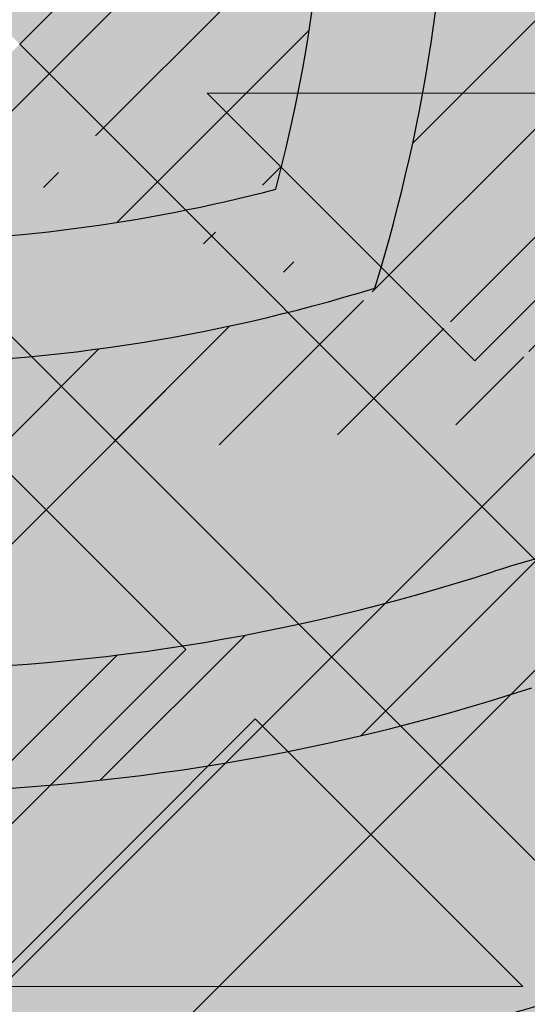
# Model space of a CAD drawing. Units: inches. Extents: x 844 to 2234, y 346 to 1084.
# Tile 10 of 93: x 1123.249 to 1124.57, y 688.619 to 691.183. Entities that reach past the tile are written whole.
import ezdxf

# ---------------------------------------------------------------- set-up
doc = ezdxf.new("R2010")
doc.units = ezdxf.units.IN
doc.header["$MEASUREMENT"] = 0
for name, color, linetype, lineweight in [('A-ANNO-DIMS', 2, 'Continuous', 18), ('furniture', 8, 'Continuous', 18), ('RA-AP-01$0$INT', 35, 'Continuous', 5)]:
    doc.layers.add(name, color=color, linetype=linetype, lineweight=lineweight)
doc.layers.add('RA-AP-01$0$FURN', color=3, linetype='Continuous')
doc.layers.add('RA-AP-01$0$WOOD', color=64, linetype='Continuous')
doc.styles.get("Standard").update_dxf_attribs({"font": 'arial.ttf'})
doc.dimstyles.get("Standard").update_dxf_attribs({"dimtxt": 6, "dimasz": 3, "dimexe": 0.18, "dimexo": 0.0625, "dimgap": 0.09, "dimtad": 0, "dimtih": 1, "dimtoh": 1, "dimdec": 1, "dimzin": 0, "dimdsep": 46, "dimlunit": 3, "dimtxsty": 'Standard', "dimblk": 'ARCHTICK', "dimcen": 0.09, "dimadec": 0, "dimazin": 0, "dimtfac": 1, "dimtdec": 1, "dimtofl": 0, "dimtmove": 0, "dimatfit": 3, "dimfxl": 1, "dimtolj": 1, "dimtzin": 0, "dimarcsym": 0})

# ---------------------------------------------------------------- blocks, each defined once
blk = doc.blocks.new('A$C18D01794')
at = {"layer": 'RA-AP-01$0$INT'}
h = blk.add_hatch(color=256, dxfattribs=at)
h.paths.add_polyline_path([(4.585917135068449, -6.356712009588271), (4.555206456959269, -6.35671200958746), (4.555206456959137, -6.387422687716308), (4.874495778835233, -6.706712009592356), (4.90520645695423, -6.676001331474049)])
h.paths.add_polyline_path([(5.255206456948813, -6.387422687716306), (5.255206456948682, -6.356712009605972), (5.224495778822613, -6.356712009605161), (4.905206456953498, -6.676001331474273), (4.935917135072151, -6.706712009592924)])
h.paths.add_polyline_path([(4.935917135072559, -6.706712009592068), (4.905206456953564, -6.737422687710376), (5.255206456951813, -7.087422687708613), (5.255206456951549, -7.026001331471008)])
h.paths.add_polyline_path([(4.555206456956399, -7.026001331471013), (4.555206456956134, -7.087422687708616), (4.905206456953821, -6.737422687710943), (4.874495778835166, -6.70671200959229)])
h = blk.add_hatch(color=256, dxfattribs=at)
h.paths.add_polyline_path([(4.585917135068448, -6.356712009588273), (4.614201406330596, -6.356712009589021), (4.668846067270487, -6.411356670531338), (4.723490728212344, -6.356712009591912), (4.771774999457151, -6.35671200959319), (4.826419660396886, -6.411356670535356), (4.862780050090322, -6.374996280843536), (4.844495778842715, -6.356712009595112), (4.862780050090411, -6.356712009595595), (4.905206456960182, -6.399138416468211), (4.947632863832445, -6.356712009597838), (4.965917135079675, -6.356712009598322), (4.947632863831759, -6.374996280845421), (4.983993253523576, -6.411356670538857), (5.038637914464627, -6.356712009600247), (5.08692218571208, -6.356712009601523), (5.141566846649976, -6.411356670541852), (5.196211507589851, -6.356712009604411), (5.224495778822615, -6.356712009605161), (4.905206456953975, -6.676001331473793)])
h.paths.add_polyline_path([(4.895206456956031, -6.637717060225675), (4.895206456958921, -6.528427738347902), (4.840561796018589, -6.583072399285802)], flags=16)
h.paths.add_polyline_path([(4.915206456955638, -6.637717060226121), (4.969851117895509, -6.583072399288678), (4.915206456957609, -6.528427738348344)], flags=16)
h.paths.add_polyline_path([(4.826419660395175, -6.568930263661755), (4.881064321335613, -6.514285602723745), (4.771774999456703, -6.514285602720857)], flags=16)
h.paths.add_polyline_path([(4.983993253519558, -6.568930263665262), (5.038637914460456, -6.514285602726792), (4.929348592581548, -6.514285602724816)], flags=16)
h.paths.add_polyline_path([(4.881064321336025, -6.494285602723742), (4.826419660397532, -6.439640941782821), (4.771774999457062, -6.494285602720859)], flags=16)
h.paths.add_polyline_path([(4.929348592582019, -6.494285602724817), (5.038637914460982, -6.494285602726792), (4.983993253522945, -6.439640941786327)], flags=16)
h.paths.add_polyline_path([(4.895206456960191, -6.480143467100443), (4.895206456962115, -6.407422687715913), (4.876922185715016, -6.389138416467584), (4.840561796021581, -6.425498806159401)], flags=16)
h.paths.add_polyline_path([(4.915206456958487, -6.480143467100889), (4.969851117899527, -6.425498806162279), (4.933490728206909, -6.389138416468043), (4.9152064569598, -6.40742268771434)], flags=16)
h.paths.add_polyline_path([(4.757632863832376, -6.480143467096812), (4.812277524772842, -6.425498806158772), (4.757632863834348, -6.370854145217844)], flags=16)
h.paths.add_polyline_path([(4.737632863832376, -6.480143467096286), (4.737632863834348, -6.370854145217375), (4.682988202893906, -6.425498806155385)], flags=16)
h.paths.add_polyline_path([(5.05278005008503, -6.480143467103376), (5.052780050087917, -6.370854145224413), (4.998135389146995, -6.425498806162908)], flags=16)
h.paths.add_polyline_path([(5.072780050085024, -6.480143467103744), (5.127424711025931, -6.42549880616527), (5.072780050087916, -6.370854145224832)], flags=16)
h.paths.add_polyline_path([(4.935917135072783, -6.706712009592292), (5.255206456948811, -6.387422687716309), (5.255206456948932, -6.415706958964177), (5.200561796010279, -6.470351619902839), (5.255206456949403, -6.524996280841948), (5.25520645694961, -6.5732805520894), (5.200561796009787, -6.627925213029239), (5.236922185702417, -6.664285602721864), (5.255206456949919, -6.646001331474357), (5.255206456949998, -6.664285602721898), (5.212780050078687, -6.706712009592262), (5.25520645695036, -6.749138416463932), (5.255206456950438, -6.767422687711313), (5.236922185702424, -6.749138416463297), (5.200561796009796, -6.785498806155928), (5.255206456950753, -6.840143467096874), (5.25520645695096, -6.888427738341682), (5.200561796010322, -6.943072399282328), (5.255206456951428, -6.997717060223427), (5.255206456951547, -7.026001331471006)])
h.paths.add_polyline_path([(5.042988202883395, -6.785498806155427), (5.097632863823085, -6.840143467095101), (5.097632863822622, -6.730854145216193)], flags=16)
h.paths.add_polyline_path([(5.028846067259663, -6.771356670531693), (5.083490728198774, -6.716712009592573), (4.974201406321001, -6.716712009593042)], flags=16)
h.paths.add_polyline_path([(5.117632863823087, -6.840143467095186), (5.172277524762331, -6.785498806155926), (5.11763286382262, -6.730854145216225)], flags=16)
h.paths.add_polyline_path([(5.08349072819877, -6.696712009593886), (5.028846067259652, -6.642067348654775), (4.974201406320998, -6.696712009593438)], flags=16)
h.paths.add_polyline_path([(5.131774999446817, -6.854285602718917), (5.186419660386065, -6.799640941779662), (5.241064321325782, -6.854285602719365)], flags=17)
h.paths.add_polyline_path([(5.131774999446228, -6.716712009592374), (5.186419660386065, -6.771356670532194), (5.222780050079488, -6.734996280838764), (5.204495778832781, -6.716712009592063)], flags=16)
h.paths.add_polyline_path([(5.097632863822613, -6.682569873970264), (5.097632863823061, -6.573280552091354), (5.042988202883383, -6.627925213031044)], flags=16)
h.paths.add_polyline_path([(5.131774999446899, -6.874285602718915), (5.241064321325809, -6.874285602719364), (5.186419660386591, -6.928930263658598)], flags=17)
h.paths.add_polyline_path([(5.131774999446226, -6.696712009594078), (5.204495778830767, -6.696712009594374), (5.22278005007868, -6.67842773834687), (5.186419660386049, -6.642067348654249)], flags=16)
h.paths.add_polyline_path([(5.11763286382262, -6.682569873970225), (5.17227752476232, -6.627925213030515), (5.117632863823064, -6.573280552091267)], flags=16)
h.paths.add_polyline_path([(5.186419660386069, -6.613783077405491), (5.241064321325754, -6.559138416465795), (5.131774999446791, -6.559138416466263)], flags=16)
h.paths.add_polyline_path([(5.131774999446872, -6.539138416466263), (5.24106432132578, -6.539138416465794), (5.186419660386554, -6.484493755526573)], flags=16)
h.paths.add_polyline_path([(5.255206456951811, -7.08742268770861), (5.255206456951895, -7.106712009588038), (4.555206456956052, -7.106712009588038), (4.555206456956136, -7.087422687708617), (4.905206456953973, -6.737422687710788)])
h.paths.add_polyline_path([(4.983993253513404, -6.8444937555241), (4.92934859257295, -6.899138416462108), (5.03863791445186, -6.899138416465014)], flags=16)
h.paths.add_polyline_path([(4.969851117889988, -6.83035161990006), (4.915206456952556, -6.775706958960171), (4.915206456949648, -6.884996280837944)], flags=16)
h.paths.add_polyline_path([(4.929348592572535, -6.919138416462105), (4.983993253511019, -6.973783077403037), (5.038637914451496, -6.919138416465012)], flags=16)
h.paths.add_polyline_path([(5.052780050074912, -6.93328055208906), (4.998135389134438, -6.987925213027088), (5.052780050072919, -7.042569873968025)], flags=16)
h.paths.add_polyline_path([(5.07278005007491, -6.933280552089588), (5.072780050072918, -7.042569873968497), (5.127424711013374, -6.987925213030498)], flags=16)
h.paths.add_polyline_path([(4.89520645695295, -6.775706958959721), (4.840561796013067, -6.830351619897157), (4.895206456950961, -6.884996280837494)], flags=16)
h.paths.add_polyline_path([(4.915206456948365, -6.933280552085403), (4.915206456946434, -7.006001331471951), (4.933490728192729, -7.024285602719066), (4.969851117886972, -6.987925213026453)], flags=16)
h.paths.add_polyline_path([(4.881064321327021, -6.899138416461022), (4.82641966038902, -6.84449375552057), (4.771774999448108, -6.899138416459029)], flags=16)
h.paths.add_polyline_path([(4.895206456950073, -6.933280552084951), (4.840561796009022, -6.987925213023558), (4.876922185700835, -7.024285602716997), (4.895206456948749, -7.006001331469487)], flags=16)
h.paths.add_polyline_path([(4.983993253510392, -7.0020673486505), (4.947632863816944, -7.038427738342319), (4.965917135064043, -7.05671200959023), (5.038637914448995, -7.056712009591555)], flags=16)
h.paths.add_polyline_path([(4.881064321326543, -6.91913841646102), (4.771774999447578, -6.919138416459031), (4.826419660385607, -6.973783077399508)], flags=16)
h.paths.add_polyline_path([(4.905206456946447, -7.014285602717636), (4.862780050074785, -7.056712009588352), (4.947632863816685, -7.056712009589775)], flags=16)
h.paths.add_polyline_path([(5.14156684663679, -7.002067348654549), (5.086922185696452, -7.056712009592438), (5.196211507574223, -7.056712009594425)], flags=16)
h.paths.add_polyline_path([(4.8264196603837, -7.002067348646972), (4.771774999442643, -7.056712009585575), (4.8444957788276, -7.056712009587508), (4.862780050075511, -7.038427738340416)], flags=16)
h.paths.add_polyline_path([(4.812277524760289, -6.98792521302292), (4.757632863822258, -6.933280552082447), (4.757632863819352, -7.042569873961408)], flags=16)
h.paths.add_polyline_path([(4.73763286382226, -6.933280552082079), (4.682988202881349, -6.987925213020536), (4.737632863819352, -7.04256987396099)], flags=16)
h.paths.add_polyline_path([(4.723490728195188, -7.056712009584289), (4.668846067257299, -7.002067348643949), (4.614201406317417, -7.056712009581383)], flags=16)
h.paths.add_polyline_path([(4.597632863829262, -6.706712009592262), (4.555206456957951, -6.664285602721896), (4.555206456958029, -6.646001331474357), (4.573490728205535, -6.664285602721864), (4.609851117898167, -6.627925213029238), (4.555206456958338, -6.573280552089402), (4.555206456958546, -6.524996280841952), (4.60985111789767, -6.470351619902839), (4.555206456959015, -6.415706958964177), (4.555206456959138, -6.387422687716309), (4.874495778835167, -6.70671200959229), (4.5552064569564, -7.026001331471015), (4.555206456956523, -6.997717060223433), (4.609851117897629, -6.94307239928233), (4.555206456956988, -6.888427738341681), (4.555206456957198, -6.840143467096881), (4.609851117898153, -6.78549880615593), (4.573490728205528, -6.749138416463297), (4.555206456957507, -6.76742268771132), (4.555206456957585, -6.749138416463933)])
h.paths.add_polyline_path([(4.712780050085332, -6.730854145216195), (4.712780050084863, -6.840143467095105), (4.767424711024555, -6.785498806155427)], flags=16)
h.paths.add_polyline_path([(4.726922185709173, -6.716712009592573), (4.781566846648288, -6.771356670531693), (4.836211507586949, -6.716712009593043)], flags=16)
h.paths.add_polyline_path([(4.692780050085327, -6.730854145216225), (4.638135389145619, -6.785498806155928), (4.692780050084865, -6.840143467095185)], flags=16)
h.paths.add_polyline_path([(4.726922185709182, -6.696712009593886), (4.836211507586949, -6.696712009593436), (4.7815668466483, -6.642067348654773)], flags=16)
h.paths.add_polyline_path([(4.678637914461726, -6.71671200959237), (4.605917135075169, -6.716712009592063), (4.587632863828464, -6.734996280838766), (4.623993253521887, -6.771356670532195)], flags=16)
h.paths.add_polyline_path([(4.712780050085336, -6.68256987397026), (4.767424711024568, -6.627925213031042), (4.71278005008489, -6.573280552091352)], flags=16)
h.paths.add_polyline_path([(4.678637914461726, -6.696712009594076), (4.623993253521899, -6.642067348654247), (4.587632863829271, -6.67842773834687), (4.605917135077185, -6.696712009594376)], flags=16)
h.paths.add_polyline_path([(4.692780050085336, -6.682569873970228), (4.692780050084889, -6.573280552091267), (4.638135389145632, -6.627925213030515)], flags=16)
h.paths.add_polyline_path([(4.623993253521885, -6.799640941779662), (4.678637914461131, -6.854285602718915), (4.56934859258217, -6.854285602719365)], flags=17)
h.paths.add_polyline_path([(4.623993253521901, -6.613783077405509), (4.678637914461158, -6.559138416466263), (4.569348592582195, -6.559138416465795)], flags=16)
h.paths.add_polyline_path([(4.678637914461051, -6.874285602718915), (4.623993253521361, -6.928930263658598), (4.569348592582143, -6.874285602719364)], flags=17)
h.paths.add_polyline_path([(4.678637914461076, -6.539138416466263), (4.623993253521399, -6.484493755526573), (4.569348592582167, -6.539138416465796)], flags=16)
h = blk.add_hatch(color=256, dxfattribs=at)
h.paths.add_polyline_path([(4.969851117891331, -6.583072399286455), (4.915206456952669, -6.63771706022511), (4.915206456952222, -6.528427738347337)])
h.paths.add_polyline_path([(4.895206456953064, -6.637717060225108), (4.840561796014413, -6.583072399286448), (4.895206456953533, -6.528427738347335)])
h.paths.add_polyline_path([(4.826419660390684, -6.568930263662714), (4.771774999451003, -6.514285602723024), (4.881064321329913, -6.514285602723489)])
h.paths.add_polyline_path([(4.881064321329884, -6.494285602723492), (4.771774999450921, -6.494285602723024), (4.82641966039018, -6.439640941783778)])
h.paths.add_polyline_path([(4.895206456953734, -6.48014346709988), (4.840561796013912, -6.425498806160046), (4.876922185707337, -6.389138416466622), (4.895206456954043, -6.40742268771333)])
h.paths.add_polyline_path([(4.862780050082808, -6.374996280843689), (4.826419660390178, -6.411356670536314), (4.771774999450351, -6.356712009596481), (4.844495778835303, -6.356712009596181)])
h.paths.add_polyline_path([(4.812277524766446, -6.425498806160041), (4.757632863827191, -6.480143467099289), (4.757632863826741, -6.370854145220329)])
h.paths.add_polyline_path([(4.737632863827191, -6.480143467099214), (4.682988202887508, -6.425498806159518), (4.737632863826743, -6.370854145220299)])
h.paths.add_polyline_path([(4.668846067263777, -6.41135667053579), (4.614201406325123, -6.356712009597128), (4.723490728202894, -6.356712009596675)])
h.paths.add_polyline_path([(4.905206456953846, -6.399138416467422), (4.862780050082654, -6.356712009596229), (4.947632863824561, -6.356712009595756)])
h.paths.add_polyline_path([(4.915206456952028, -6.480143467099882), (4.91520645695173, -6.407422687715346), (4.933490728199234, -6.389138416467428), (4.96985111789186, -6.425498806160055)])
h.paths.add_polyline_path([(5.038637914454841, -6.494285602723048), (4.929348592575874, -6.494285602723497), (4.983993253515593, -6.439640941783787)])
h.paths.add_polyline_path([(4.983993253515065, -6.568930263662725), (4.929348592575849, -6.514285602723495), (5.038637914454755, -6.514285602723045)])
h.paths.add_polyline_path([(5.052780050079843, -6.480143467099317), (4.998135389140595, -6.425498806160058), (5.052780050080309, -6.370854145220356)])
h.paths.add_polyline_path([(4.983993253516868, -6.411356670536324), (4.947632863824241, -6.374996280843694), (4.965917135071747, -6.356712009596188), (5.038637914456701, -6.356712009596504)])
h.paths.add_polyline_path([(5.127424711019533, -6.425498806159557), (5.072780050079843, -6.480143467099239), (5.07278005008031, -6.370854145220326)])
h.paths.add_polyline_path([(5.141566846643269, -6.411356670535829), (5.086922185704154, -6.356712009596707), (5.196211507581929, -6.356712009597176)])
h = blk.add_hatch(color=256, dxfattribs=at)
h.paths.add_polyline_path([(5.028846067259997, -6.642067348655121), (4.974201406321342, -6.696712009593783), (5.083490728199115, -6.69671200959423)])
h.paths.add_polyline_path([(4.974201406321344, -6.716712009593388), (5.028846067260004, -6.771356670532039), (5.083490728199117, -6.716712009592919)])
h.paths.add_polyline_path([(5.042988202883738, -6.785498806155768), (5.097632863823428, -6.840143467095449), (5.097632863822963, -6.73085414521654)])
h.paths.add_polyline_path([(5.117632863822961, -6.730854145216568), (5.117632863823428, -6.840143467095531), (5.172277524762674, -6.785498806156272)])
h.paths.add_polyline_path([(5.131774999446572, -6.716712009592718), (5.186419660386406, -6.77135667053254), (5.222780050079831, -6.734996280839116), (5.204495778833122, -6.716712009592409)])
h.paths.add_polyline_path([(5.236922185702764, -6.749138416463644), (5.200561796010139, -6.785498806156274), (5.255206456949971, -6.840143467096101), (5.255206456950271, -6.76742268771115)])
h.paths.add_polyline_path([(5.186419660386412, -6.799640941780006), (5.131774999447164, -6.854285602719262), (5.241064321326123, -6.854285602719711)])
h.paths.add_polyline_path([(5.131774999447238, -6.874285602719261), (5.186419660386934, -6.928930263658944), (5.241064321326153, -6.874285602719709)])
h.paths.add_polyline_path([(5.200561796010663, -6.943072399282675), (5.255206456949324, -6.997717060221329), (5.255206456949777, -6.888427738343558)])
h.paths.add_polyline_path([(5.21278005007903, -6.706712009592607), (5.255206456950223, -6.749138416463798), (5.255206456950696, -6.664285602721891)])
h.paths.add_polyline_path([(5.13177499944657, -6.696712009594424), (5.204495778831106, -6.696712009594723), (5.222780050079024, -6.678427738347219), (5.186419660386397, -6.642067348654592)])
h.paths.add_polyline_path([(5.117632863823405, -6.573280552091611), (5.117632863822955, -6.682569873970578), (5.172277524762665, -6.627925213030859)])
h.paths.add_polyline_path([(5.042988202883727, -6.627925213031387), (5.097632863822957, -6.682569873970603), (5.097632863823407, -6.573280552091697)])
h.paths.add_polyline_path([(5.131774999447135, -6.559138416466609), (5.186419660386394, -6.613783077405857), (5.241064321326097, -6.559138416466144)])
h.paths.add_polyline_path([(5.200561796010128, -6.627925213029584), (5.236922185702758, -6.664285602722211), (5.255206456950264, -6.646001331474705), (5.255206456949948, -6.573280552089752)])
h.paths.add_polyline_path([(5.186419660386895, -6.484493755526919), (5.131774999447213, -6.539138416466609), (5.241064321326127, -6.539138416466142)])
h.paths.add_polyline_path([(5.200561796010624, -6.470351619903183), (5.255206456949745, -6.524996280842298), (5.255206456949276, -6.415706958964523)])
for p, q in [((4.905206456953975, -6.676001331473793), (5.224495778822613, -6.356712009605161)), ((4.935917135072783, -6.706712009592292), (5.255206456948813, -6.387422687716307)), ((4.929348592581546, -6.514285602724816), (4.983993253519556, -6.568930263665262)), ((5.038637914460456, -6.514285602726792), (4.929348592581546, -6.514285602724816)), ((4.983993253519558, -6.56893026366526), (5.038637914460456, -6.514285602726792)), ((4.915206456957613, -6.52842773834835), (4.969851117895507, -6.583072399288678)), ((4.915206456955636, -6.637717060226119), (4.969851117895507, -6.583072399288678)), ((4.974201406320999, -6.696712009593436), (5.028846067259652, -6.642067348654775)), ((5.083490728198769, -6.696712009593882), (5.028846067259652, -6.642067348654775)), ((5.08349072819877, -6.696712009593886), (4.974201406320999, -6.696712009593436)), ((4.935917135072783, -6.706712009592292), (5.255206456951548, -7.026001331471007))]:
    blk.add_line(p, q, dxfattribs=at)
blk = doc.blocks.new('A$C32926AE1')
at = {"layer": 'RA-AP-01$0$FURN'}
h = blk.add_hatch(dxfattribs=at)
h.set_pattern_fill('ANSI31', color=256, scale=0.1, style=0)
h.set_pattern_definition([(45, (0, 0), (-0.0088388347648318, 0.0088388347648318), [])])
edge = h.paths.add_edge_path(flags=16)
edge.add_arc((4.904771284329206, 4.246793130718756), 0.2603971832811541, 75.22398030683196, 104.7760196931204)
edge.add_arc((4.904771284329206, 4.246793130718756), 0.2603971832811541, 75.223980306832, 104.77601969312039, ccw=False)
edge = h.paths.add_edge_path(flags=16)
edge.add_arc((4.904771284329206, 4.067062675376612), 0.2603971832811541, 255.2239803068796, 284.776019693168)
edge.add_arc((4.904771284329206, 4.067062675376612), 0.2603971832811541, 255.22398030687958, 284.77601969316805, ccw=False)
edge = h.paths.add_edge_path(flags=0)
edge.add_arc((4.904771284329206, 4.067062675376612), 0.2603971832811541, 255.2239803068796, 284.776019693168)
edge.add_arc((4.904771284329206, 4.067062675376612), 0.2603971832811541, 255.22398030687958, 284.77601969316805, ccw=False)
edge = h.paths.add_edge_path(flags=0)
edge.add_arc((4.904771284329206, 4.067062675376612), 0.2603971832811541, 255.2239803068796, 284.776019693168)
edge.add_arc((4.904771284329206, 4.067062675376612), 0.2603971832811541, 255.22398030687958, 284.77601969316805, ccw=False)
edge = h.paths.add_edge_path()
edge.add_arc((4.604388392048174, 4.588829985554312), 0.1599999999999918, 342.3781640246255, 354.4317409793762)
edge.add_arc((5.090145208887507, 4.43216705527679), 0.3503971832811637, 162.0091218307731, 180.3186872093483)
edge.add_arc((5.205154176610243, 4.588829985554953), 0.1599999999999917, 185.5682590208461, 197.6218359767349)
edge.add_arc((4.904771284329229, 4.246793130718735), 0.3503971832811761, 72.00912183053516, 107.9908781690354)
edge.add_arc((9.535952835716557, 4.28682295566602), 4.798342501046485, 178.2875002453811, 181.5576802719453)
edge.add_arc((4.719397359771122, 4.43216705527679), 0.3503971832811637, 359.6813127906516, 377.9908781692269)
edge.add_arc((9.535967292294904, 4.286822350292874), 4.778371420254705, 178.2965938931842, 181.5667745797229)
edge.add_arc((4.719397359771122, 4.43216705527679), 0.3303971832811637, 359.6813127906516, 377.9908781692269)
edge.add_arc((0.2735752763637294, 4.286822350292874), 4.7783714202547, 358.4332254202771, 361.7034061068158)
edge.add_arc((5.061434214606998, 4.732549947558029), 0.1600000000000254, 252.3781640250584, 264.4317409792362)
edge.add_arc((4.748108354051257, 4.732549947558012), 0.1600000000000541, 275.5682590208426, 287.6218359759532)
edge.add_arc((4.604388392048115, 4.588829985554317), 0.1800000000000505, 342.3567572500182, 349.3735009646207)
edge.add_arc((5.205154176610254, 4.588829985554976), 0.1800000000000069, 190.6264990356027, 197.6432427513933)
edge.add_arc((5.061434214607106, 4.732549947558013), 0.1800000000000424, 252.3567572496606, 259.3735009644582)
edge.add_arc((4.904771284329208, 4.246793130718737), 0.3303971832811676, 71.99844483668534, 108.0015551637021)
edge.add_arc((4.748108354051414, 4.732549947558045), 0.1800000000000547, 280.6264990355479, 287.6432427495938)
edge.add_arc((5.090145208887514, 4.432167055276789), 0.2803971832811691, 162.8706300666893, 180.816523289902)
edge.add_arc((4.719397359771136, 4.432167055276689), 0.2803971832811534, 359.183476710103, 377.1293699333214)
edge.add_arc((4.904771284329222, 4.246793130718737), 0.2803971832811769, 72.87063006672916, 107.1293699332334)
edge.add_arc((5.090145208887522, 4.432167055276788), 0.2603971832811776, 165.2239803068007, 180.9953123810312)
edge.add_arc((4.719397359771141, 4.432167055276699), 0.2603971832811458, 359.0046876189768, 374.7760196932087)
edge.add_arc((5.090145208887507, 4.43216705527679), 0.3303971832811637, 162.0091218307731, 180.3186872093483)
edge.add_arc((9.53595427642584, 4.285015535491528), 4.728345371032053, 178.265043920078, 181.5679956281801)
edge.add_arc((0.2735882922327999, 4.285015535491582), 4.728345371032045, 358.4320043718193, 361.7349560799204)
edge.add_arc((9.535953591267507, 4.284458026472751), 4.708343996644348, 178.2573054306777, 181.5704995759608)
edge.add_arc((0.273588977391114, 4.284458026472785), 4.708343996644358, 358.4295004240388, 361.7426945693213)
edge.add_arc((0.2735889773911131, 4.029397779622582), 4.708343996644359, 358.2573054306787, 361.5704995759613)
edge.add_arc((9.535953591267518, 4.029397779622618), 4.708343996644359, 178.4295004240391, 181.7426945693223)
edge.add_arc((0.2735882922327901, 4.028840270603786), 4.728345371032054, 358.2650439200796, 361.5679956281808)
edge.add_arc((9.53595427642584, 4.028840270603841), 4.728345371032054, 178.4320043718199, 181.7349560799219)
edge.add_arc((0.2735752763637302, 4.027033455802493), 4.778371420254699, 358.2965938931842, 361.5667745797229)
edge.add_arc((4.719397359771122, 3.881688750818578), 0.3303971832811637, 342.0091218307731, 360.3186872093484)
edge.add_arc((5.090145208887507, 3.881688750818578), 0.3303971832811637, 179.6813127906516, 197.9908781692269)
edge.add_arc((9.535967292294904, 4.027033455802493), 4.778371420254705, 178.433225420277, 181.7034061068158)
edge.add_arc((4.719397359771122, 3.881688750818578), 0.3503971832811637, 342.0091218307731, 360.3186872093484)
edge.add_arc((9.53595283571655, 4.027032850429349), 4.79834250104648, 178.4423197280546, 181.7124997546188)
edge.add_arc((4.719397359771141, 3.881688750818669), 0.2603971832811458, 345.2239803067913, 360.9953123810232)
edge.add_arc((5.090145208887522, 3.88168875081858), 0.2603971832811776, 179.0046876189687, 194.7760196931993)
edge.add_arc((4.904771284329222, 4.067062675376631), 0.2803971832811769, 252.8706300667665, 287.1293699332708)
edge.add_arc((4.719397359771136, 3.881688750818678), 0.2803971832811534, 342.8706300666787, 360.8165232898969)
edge.add_arc((5.090145208887514, 3.881688750818579), 0.2803971832811691, 179.183476710098, 197.1293699333106)
edge.add_arc((4.748108354051414, 3.581305858537323), 0.1800000000000547, 72.3567572504062, 79.37350096445199)
edge.add_arc((4.904771284329208, 4.067062675376631), 0.3303971832811676, 251.9984448362979, 288.0015551633146)
edge.add_arc((5.061434214607106, 3.581305858537355), 0.1800000000000424, 100.6264990355418, 107.6432427503394)
edge.add_arc((5.205154176610254, 3.725025820540392), 0.1800000000000069, 162.3567572486066, 169.3735009643972)
edge.add_arc((4.604388392048115, 3.725025820541051), 0.1800000000000505, 10.62649903537925, 17.64324274998182)
edge.add_arc((4.748108354051257, 3.581305858537356), 0.1600000000000541, 72.37816402404681, 84.43174097915735)
edge.add_arc((4.904771284329229, 4.067062675376632), 0.3503971832811761, 252.0091218309645, 287.9908781694648)
edge.add_arc((5.061434214606998, 3.581305858537339), 0.1600000000000254, 95.56825902076373, 107.6218359749416)
edge.add_arc((5.205154176610243, 3.725025820540414), 0.1599999999999917, 162.3781640232651, 174.4317409791539)
edge.add_arc((5.090145208887507, 3.881688750818578), 0.3503971832811637, 179.6813127906516, 197.9908781692269)
edge.add_arc((4.604388392048174, 3.725025820541056), 0.1599999999999918, 5.568259020623824, 17.62183597537444)
edge.add_arc((0.2735897329420762, 4.28682295566602), 4.798342501046482, 358.4423197280547, 361.7124997546188)
edge.add_arc((0.2735897329420691, 4.027032850429348), 4.798342501046489, 358.2875002453812, 361.5576802719453)
at = {"layer": 'RA-AP-01$0$WOOD'}
h = blk.add_hatch(color=256, dxfattribs=at)
h.dxf.hatch_style = 1
h.paths.add_polyline_path([(5.157430609644524, 4.573483066760929, -0.1009492694046607), (5.155401577623758, 4.593365984175333, -0.1842662638101597), (5.172249623284174, 4.638795604568598, 0.2056608120311276), (5.179560981299304, 4.661316324430096, 0.3614336704623542), (5.134352340494423, 4.706524965234944, 0.2056608120311297), (5.111831620632933, 4.699213607219793, -0.1842662638101113), (5.066402000239693, 4.682365561559342, -0.1055311479399994), (5.045656153913092, 4.68467289944697, 0.1567636581983829), (4.763886414745334, 4.684672899446966, -0.1055311479399895), (4.743140568418733, 4.68236556155934, -0.1842662638100833), (4.6977109480255, 4.69921360721979, 0.2056608120302612), (4.675190228164109, 4.706524965234949, 0.3614336704708441), (4.629981587358889, 4.66131632442871, 0.2056608120245944), (4.637292945374126, 4.638795604567974, -0.1842662638101024), (4.654140991034615, 4.59336598417475, -0.1009492694055169), (4.652111959013835, 4.573483066760181, 0.021410119221476), (4.629748025606143, 4.156712009541676, 0.0214101192214795), (4.652111959013809, 3.739940952323101, -0.1009492694059586), (4.654140991034615, 3.720058034908448, -0.1842662638100975), (4.637292945374126, 3.674628414515226, 0.2056608120245705), (4.629981587358889, 3.652107694654492, 0.3614336704708879), (4.675190228164113, 3.606899053848249, 0.2056608120302384), (4.697710948025501, 3.614210411863408, -0.1842662638100995), (4.743140568418738, 3.63105845752386, -0.1055311479402541), (4.763886414745388, 3.628751119636215, 0.1567636581983776), (5.045656153913137, 3.628751119636244, -0.1055311479397538), (5.066402000239692, 3.631058457523857, -0.1842662638101067), (5.111831620632931, 3.614210411863407, 0.2056608120310924), (5.134352340494417, 3.606899053848256, 0.3614336704624001), (5.179560981299307, 3.652107694653103, 0.2056608120311314), (5.172249623284175, 3.6746284145146, -0.1842662638101402), (5.155401577623758, 3.72005803490786, -0.1009492694051366), (5.15743060964455, 3.739940952322354, 0.0214101192215073), (5.179794543052287, 4.156712009541468, 0.0214101192215252)])
h.paths.add_polyline_path([(4.639748609479751, 4.156712009541513, 0.0213537860821624), (4.661970494867118, 3.741887061152232, -0.094075836301374), (4.664143710413708, 3.7196126951003, -0.1824818158568985), (4.644813765429836, 3.668037719127816, 0.2056608120245319), (4.639939526753007, 3.653023905887301, 0.3614336704710246), (4.676106439397173, 3.616856993242342, 0.2056608120302234), (4.691120252638095, 3.621731231919122, -0.1824818158602558), (4.742695228611606, 3.641061176902986, -0.1029891339458722), (4.766991894714349, 3.638256818950944, 0.156709409989566), (5.042550673941472, 3.638256818950105, -0.102989133958497), (5.066847340047078, 3.641061176902949, -0.1824818158594995), (5.118422316020358, 3.621731231919103, 0.2056608120311416), (5.133436129261316, 3.616856993242346, 0.3614336704621468), (5.169603041905217, 3.653023905886178, 0.2056608120310986), (5.164728803228477, 3.668037719127177, -0.1824818158565612), (5.145398858244737, 3.719612695099578, -0.0940758363009313), (5.147572073791232, 3.741887061151398, 0.0213537860822023), (5.169793959178681, 4.156712009541451, 0.0213537860822226), (5.147572073791203, 4.571536957931898, -0.0940758363005034), (5.145398858244737, 4.59381132398362, -0.1824818158565587), (5.164728803228476, 4.645386299956021, 0.2056608120311045), (5.169603041905216, 4.66040011319702, 0.3614336704621845), (5.133436129261313, 4.696567025840856, 0.2056608120310773), (5.118422316020359, 4.691692787164098, -0.182481815859508), (5.066847340047078, 4.67236284218025, -0.1029891339584606), (5.04255067394148, 4.675167200133092, 0.156709409989566), (4.766991894714357, 4.675167200132257, -0.1029891339458842), (4.742695228611611, 4.672362842180213, -0.1824818158602725), (4.691120252638095, 4.691692787164077, 0.2056608120302152), (4.676106439397174, 4.696567025840858, 0.3614336704710363), (4.639939526753005, 4.660400113195899, 0.2056608120245495), (4.644813765429837, 4.645386299955384, -0.1824818158568934), (4.664143710413708, 4.593811323982902, -0.0940758363009187), (4.661970494867149, 4.571536957931074, 0.021353786082177)], flags=16)
h.paths.add_polyline_path([(5.129794543052235, 4.432167055276933, -0.0141661062790638), (5.130152669293814, 4.156927903047693, -0.0141661062790647), (5.129794543052234, 3.881688750818433, -0.0785247771143638), (5.10979738006795, 3.755143611847103, 0.0945969212073497), (5.105408519571111, 3.717898134952927, 0.1043170707844957), (5.116074640131521, 3.670385395016088, 0.1043170707864965), (5.068561900193738, 3.681051515576561, 0.09459692119553), (5.031316423304057, 3.676662655080835, -0.1580239521427272), (4.778226145355827, 3.676662655080367, 0.0945969211986668), (4.740980668464973, 3.681051515576592, 0.1043170707882822), (4.693467928526415, 3.670385395015844, 0.1043170707867916), (4.704134049087309, 3.717898134953662, 0.0945969211972894), (4.69974518859162, 3.755143611844042, -0.0785247771163196), (4.679748025606343, 3.881688750818406, -0.0141661062790663), (4.679389899364763, 4.156927903047693, -0.0141661062790672), (4.679748025606343, 4.432167055276998, -0.0785247771163064), (4.699745188591625, 4.55871219425134, 0.094596921197333), (4.704134049087308, 4.595957671141738, 0.1043170707867205), (4.693467928526416, 4.643470411079523, 0.1043170707882628), (4.740980668464965, 4.632804290518776, 0.0945969211988114), (4.778226145355874, 4.637193151015016, -0.158023952142669), (5.031316423304015, 4.637193151014546, 0.0945969211956361), (5.068561900193736, 4.632804290518806, 0.1043170707864979), (5.11607464013152, 4.643470411079278, 0.1043170707844617), (5.105408519571112, 4.595957671142455, 0.0945969212074597), (5.109797380067959, 4.558712194248236, -0.0785247771143467)], flags=0)
h.paths.add_polyline_path([(5.119794532311105, 4.432259799204851, -0.0142000800617244), (5.120156169157484, 4.156927903047701, -0.0142000800617277), (5.119794532311105, 3.881596006890482, -0.0784894509520253), (5.100273383573699, 3.758192358677797, 0.0940138827242913), (5.095413455884425, 3.717477693979438, 0.0606271852308753), (5.099615656341024, 3.686844378806616, 0.0606271852322524), (5.068982341167493, 3.691046579263239, 0.0940138827010453), (5.028267676478798, 3.686186651576848, -0.1580706864508061), (4.781274892180912, 3.686186651576435, 0.0940138827026903), (4.740560227491556, 3.691046579263279, 0.0606271852339895), (4.709926912317155, 3.686844378806508, 0.0606271852329405), (4.714129112773991, 3.717477693980356, 0.094013882701304), (4.709269185087677, 3.758192358669163, -0.0784894509577193), (4.689748036347473, 3.881596006890469, -0.014200080061729), (4.689386399501094, 4.156927903047709, -0.0142000800617217), (4.689748036347473, 4.432259799204808, -0.078489450957724), (4.709269185087651, 4.555663447426125, 0.0940138827014585), (4.714129112773992, 4.596378112114996, 0.0606271852329731), (4.709926912317154, 4.62701142728886, 0.0606271852340196), (4.74056022749157, 4.622809226832087, 0.0940138827024997), (4.781274892180847, 4.627669154518912, -0.1580706864508359), (5.028267676478777, 4.627669154518526, 0.0940138827010946), (5.068982341167492, 4.622809226832129, 0.060627185232254), (5.099615656341024, 4.627011427288751, 0.0606271852308727), (5.095413455884425, 4.59637811211593, 0.0940138827241088), (5.100273383573675, 4.555663447417647, -0.0784894509520978)], flags=0)
h.paths.add_polyline_path([(5.06978912287499, 4.430218106756144, -0.014241683694547), (5.070173729147532, 4.156927903047672, -0.0142416836945458), (5.06978912287499, 3.883637699339223, -0.0800609523125196), (5.052662118612511, 3.773463122773442, 0.0526421978001116), (5.04590916754064, 3.740550867606997, 0.0526421977992423), (5.012996912374707, 3.73379791653534, -0.1583028414718258), (4.796545656286308, 3.73379791653451, 0.0526421978034211), (4.763633401117837, 3.740550867607021, 0.0526421978018622), (4.756880450045755, 3.773463122774558, -0.0800609523117106), (4.739753445783639, 3.883637699339268, -0.0142416836945435), (4.739368839511098, 4.156927903047671, -0.0142416836945477), (4.739753445783639, 4.430218106756155, -0.0800609523116345), (4.75688045004574, 4.540392683320762, 0.052642197801941), (4.763633401117837, 4.573304938488346, 0.0526421978035071), (4.796545656286361, 4.580057889560873, -0.1583028414717561), (5.012996912374669, 4.580057889560039, 0.0526421977993048), (5.04590916754064, 4.57330493848837, 0.0526421978002057), (5.052662118612529, 4.540392683321868, -0.080060952312477)], flags=0)
h.paths.add_polyline_path([(5.049789715110557, 4.43038092723357, -0.0143097550741839), (5.05018085590259, 4.156927903047715, -0.0143097550741854), (5.049789715110558, 3.883474878861827, -0.0800685599149176), (5.03362098255317, 3.779581877367999, 0.0306258898956367), (5.028241146483733, 3.758218888663947, 0.0306258898977031), (5.006878157778253, 3.75283905259408, -0.1583983521624096), (4.802664410878162, 3.752839052594731, 0.0306258898946014), (4.781301422174808, 3.758218888663924, 0.0306258898967912), (4.775921586105202, 3.779581877368794, -0.080068559914251), (4.759752853548071, 3.883474878861786, -0.0143097550741854), (4.759361712756037, 4.156927903047671, -0.0143097550741854), (4.759752853548071, 4.430380927233557, -0.0800685599142479), (4.775921586105193, 4.534273928726546, 0.0306258898968306), (4.781301422174808, 4.555636917431444, 0.0306258898945754), (4.802664410878143, 4.561016753500631, -0.1583983521624168), (5.006878157778244, 4.561016753501291, 0.0306258898977177), (5.028241146483733, 4.555636917431421, 0.0306258898958182), (5.03362098255321, 4.534273928727244, -0.080068559914796)], flags=0)
h.paths.add_polyline_path([(4.999766070382627, 4.428171244713864, -0.0143443147609634), (5.000198441819402, 4.156927903047689, -0.0143443147609612), (4.999766070382627, 3.885684561381556, -0.0784641635803329), (4.987356730658798, 3.799103304488872, -0.1506053783831347), (4.822185837999821, 3.79910330448882, -0.0784641635803318), (4.809776498276007, 3.885684561381509, -0.014344314760963), (4.809344126839227, 4.156927903047677, -0.0143443147609645), (4.809776498276007, 4.428171244713873, -0.0784641635803192), (4.822185837999822, 4.514752501606549, -0.1506053783831338), (4.987356730658798, 4.514752501606494, -0.078464163580285)], flags=0)
h.paths.add_polyline_path([(4.979755254238824, 4.42764379880488, -0.0143772539198268), (4.980205517789977, 4.156927903047693, -0.0143772539198275), (4.979755254238824, 3.886212007290489, -0.0689242507424422), (4.971183264704897, 3.815276770442801, -0.1296645318904179), (4.838359303953726, 3.815276770442746, -0.0689242507424186), (4.829787314419809, 3.886212007290419, -0.0143772539198292), (4.829337050868653, 4.156927903047653, -0.0143772539198325), (4.829787314419809, 4.427643798804946, -0.0689242507424211), (4.838359303953725, 4.498579035652621, -0.1296645318904187), (4.971183264704897, 4.498579035652565, -0.0689242507424401)], flags=0)
h = blk.add_hatch(color=256, dxfattribs=at)
h.dxf.hatch_style = 1
h.paths.add_polyline_path([(5.145398858244737, 4.59381132398362, -0.1824818158565616), (5.164728803228476, 4.645386299956021, 0.2056608120311045), (5.169603041905216, 4.66040011319702, 0.3614336704621845), (5.133436129261313, 4.696567025840856, 0.2056608120310773), (5.118422316020359, 4.691692787164098, -0.182481815859508), (5.066847340047078, 4.67236284218025, -0.1029891339584606), (5.04255067394148, 4.675167200133092, 0.156709409989566), (4.766991894714357, 4.675167200132257, -0.1029891339458842), (4.742695228611611, 4.672362842180213, -0.1824818158602725), (4.691120252638095, 4.691692787164077, 0.2056608120302152), (4.676106439397174, 4.696567025840858, 0.3614336704710363), (4.639939526753005, 4.660400113195899, 0.2056608120245495), (4.644813765429837, 4.645386299955384, -0.1824818158568934), (4.664143710413708, 4.593811323982902, -0.0940758363009187), (4.661970494867149, 4.571536957931074, 0.0213537860821772), (4.639748609479751, 4.156712009541507, 0.0213537860821625), (4.661970494867119, 3.741887061152226, -0.0940758363013071), (4.664143710413708, 3.719612695100309, -0.1824818158569294), (4.644813765429836, 3.668037719127816, 0.2056608120245319), (4.639939526753007, 3.653023905887301, 0.3614336704710246), (4.676106439397173, 3.616856993242342, 0.2056608120302234), (4.691120252638095, 3.621731231919122, -0.1824818158602558), (4.742695228611606, 3.641061176902986, -0.1029891339458722), (4.766991894714349, 3.638256818950944, 0.156709409989566), (5.042550673941472, 3.638256818950105, -0.102989133958497), (5.066847340047078, 3.641061176902949, -0.1824818158594995), (5.118422316020358, 3.621731231919103, 0.2056608120311416), (5.133436129261316, 3.616856993242346, 0.3614336704621468), (5.169603041905217, 3.653023905886178, 0.2056608120310986), (5.164728803228477, 3.668037719127177, -0.1824818158565612), (5.145398858244737, 3.719612695099578, -0.0940758363009313), (5.147572073791232, 3.741887061151398, 0.0213537860822023), (5.169793959178681, 4.156712009541451, 0.0213537860822226), (5.147572073791203, 4.571536957931898, -0.0940758363004996)])
h.paths.add_polyline_path([(5.109797380067958, 4.55871219424824, -0.0785247771143472), (5.129794543052234, 4.432167055276936, -0.0141661062790644), (5.130152669293814, 4.156927903047685, -0.014166106279066), (5.129794543052234, 3.881688750818401, -0.0785247771143517), (5.109797380067946, 3.755143611847092, 0.0945969212073132), (5.105408519571111, 3.717898134952929, 0.1043170707844995), (5.116074640131521, 3.670385395016088, 0.1043170707864965), (5.068561900193738, 3.681051515576561, 0.09459692119553), (5.031316423304057, 3.676662655080835, -0.1580239521427272), (4.778226145355827, 3.676662655080367, 0.0945969211986668), (4.740980668464973, 3.681051515576592, 0.1043170707882822), (4.693467928526415, 3.670385395015844, 0.1043170707867916), (4.704134049087309, 3.717898134953662, 0.0945969211972894), (4.69974518859162, 3.755143611844042, -0.0785247771163196), (4.679748025606343, 3.881688750818406, -0.0141661062790663), (4.679389899364763, 4.156927903047693, -0.0141661062790672), (4.679748025606343, 4.432167055276998, -0.0785247771163064), (4.699745188591625, 4.55871219425134, 0.094596921197333), (4.704134049087308, 4.595957671141738, 0.1043170707867205), (4.693467928526416, 4.643470411079523, 0.1043170707882628), (4.740980668464965, 4.632804290518776, 0.0945969211988114), (4.778226145355874, 4.637193151015016, -0.158023952142669), (5.031316423304015, 4.637193151014546, 0.0945969211956361), (5.068561900193736, 4.632804290518806, 0.1043170707864979), (5.11607464013152, 4.643470411079278, 0.1043170707844617), (5.105408519571112, 4.595957671142455, 0.0945969212074504)], flags=16)
h.paths.add_polyline_path([(5.100273383573655, 4.55566344741771, -0.0784894509521388), (5.119794532311105, 4.432259799204852, -0.0142000800617252), (5.120156169157484, 4.156927903047686, -0.014200080061726), (5.119794532311105, 3.881596006890502, -0.0784894509520446), (5.100273383573696, 3.758192358677786, 0.0940138827242721), (5.095413455884425, 3.717477693979436, 0.0606271852308692), (5.099615656341024, 3.686844378806616, 0.0606271852322522), (5.068982341167493, 3.691046579263239, 0.0940138827010453), (5.028267676478798, 3.686186651576848, -0.1580706864508061), (4.781274892180912, 3.686186651576435, 0.0940138827026903), (4.740560227491556, 3.691046579263279, 0.0606271852339895), (4.709926912317155, 3.686844378806508, 0.0606271852329405), (4.714129112773991, 3.717477693980356, 0.094013882701304), (4.709269185087677, 3.758192358669163, -0.0784894509577193), (4.689748036347473, 3.881596006890469, -0.014200080061729), (4.689386399501094, 4.156927903047709, -0.0142000800617217), (4.689748036347473, 4.432259799204808, -0.078489450957724), (4.709269185087651, 4.555663447426125, 0.0940138827014585), (4.714129112773992, 4.596378112114996, 0.0606271852329731), (4.709926912317154, 4.62701142728886, 0.0606271852340196), (4.74056022749157, 4.622809226832087, 0.0940138827024997), (4.781274892180847, 4.627669154518912, -0.1580706864508359), (5.028267676478777, 4.627669154518526, 0.0940138827010946), (5.068982341167492, 4.622809226832129, 0.060627185232254), (5.099615656341024, 4.627011427288751, 0.0606271852308727), (5.095413455884425, 4.59637811211593, 0.094013882723957)], flags=0)
h.paths.add_polyline_path([(5.04590916754064, 4.57330493848837, 0.0526421978002057), (5.052662118612529, 4.540392683321868, -0.0800609523124783), (5.06978912287499, 4.430218106756142, -0.0142416836945469), (5.070173729147532, 4.156927903047672, -0.0142416836945458), (5.06978912287499, 3.883637699339223, -0.0800609523125196), (5.052662118612511, 3.773463122773442, 0.0526421978001116), (5.04590916754064, 3.740550867606997, 0.0526421977992423), (5.012996912374707, 3.73379791653534, -0.1583028414718258), (4.796545656286308, 3.73379791653451, 0.0526421978034211), (4.763633401117837, 3.740550867607021, 0.0526421978018622), (4.756880450045755, 3.773463122774558, -0.0800609523117106), (4.739753445783639, 3.883637699339268, -0.0142416836945435), (4.739368839511098, 4.156927903047671, -0.0142416836945477), (4.739753445783639, 4.430218106756155, -0.0800609523116345), (4.75688045004574, 4.540392683320762, 0.052642197801941), (4.763633401117837, 4.573304938488346, 0.0526421978035071), (4.796545656286361, 4.580057889560873, -0.1583028414717561), (5.012996912374669, 4.580057889560039, 0.0526421977993048)], flags=0)
h.paths.add_polyline_path([(5.028241146483733, 4.555636917431422, 0.0306258898956949), (5.033620982553182, 4.534273928727329, -0.0800685599148649), (5.049789715110557, 4.430380927233569, -0.0143097550741839), (5.05018085590259, 4.156927903047715, -0.0143097550741854), (5.049789715110558, 3.883474878861827, -0.0800685599149176), (5.03362098255317, 3.779581877367999, 0.0306258898956367), (5.028241146483733, 3.758218888663947, 0.0306258898977031), (5.006878157778253, 3.75283905259408, -0.1583983521624096), (4.802664410878162, 3.752839052594731, 0.0306258898946014), (4.781301422174808, 3.758218888663924, 0.0306258898967912), (4.775921586105202, 3.779581877368794, -0.080068559914251), (4.759752853548071, 3.883474878861786, -0.0143097550741854), (4.759361712756037, 4.156927903047671, -0.0143097550741854), (4.759752853548071, 4.430380927233557, -0.0800685599142479), (4.775921586105193, 4.534273928726546, 0.0306258898968306), (4.781301422174808, 4.555636917431444, 0.0306258898945754), (4.802664410878143, 4.561016753500631, -0.1583983521624168), (5.006878157778244, 4.561016753501291, 0.0306258898977174)], flags=0)
h.paths.add_polyline_path([(4.987356730658798, 4.514752501606494, -0.0784641635803018), (4.999766070382627, 4.428171244713845, -0.0143443147609637), (5.000198441819402, 4.156927903047665, -0.0143443147609622), (4.999766070382628, 3.885684561381514, -0.0784641635802952), (4.987356730658797, 3.799103304488872, -0.1506053783831338), (4.822185837999821, 3.799103304488819, -0.0784641635803342), (4.809776498276007, 3.885684561381512, -0.0143443147609628), (4.809344126839227, 4.156927903047676, -0.0143443147609646), (4.809776498276007, 4.428171244713873, -0.0784641635803192), (4.822185837999822, 4.514752501606549, -0.1506053783831338)], flags=0)
h.paths.add_polyline_path([(4.971183264704897, 4.498579035652566, -0.0689242507424384), (4.979755254238824, 4.427643798804883, -0.0143772539198276), (4.980205517789977, 4.15692790304768, -0.0143772539198258), (4.979755254238823, 3.88621200729051, -0.0689242507424628), (4.971183264704897, 3.815276770442801, -0.129664531890417), (4.838359303953726, 3.815276770442746, -0.0689242507424186), (4.829787314419809, 3.886212007290419, -0.0143772539198292), (4.829337050868653, 4.156927903047653, -0.0143772539198325), (4.829787314419809, 4.427643798804946, -0.0689242507424211), (4.838359303953725, 4.498579035652621, -0.1296645318904187)], flags=0)
h = blk.add_hatch(dxfattribs=at)
h.set_pattern_fill('ANSI31', color=256, scale=0.05, style=0)
h.set_pattern_definition([(45, (0, 0), (-0.0044194173824159, 0.0044194173824159), [])])
h.paths.add_polyline_path([(5.130152669293814, 4.156927903047704, 0.0141661062790657), (5.129794543052234, 4.432167055276982, 0.0777827904001433), (5.110168979996553, 4.557559993161921, -0.0976515123401879), (5.105408519571111, 4.595957671142454, -0.1043170707844687), (5.116074640131522, 4.64347041107928), (5.099615656341024, 4.627011427288751, 0.0606271852308727), (5.095413455884425, 4.59637811211593, 0.0940138827241088), (5.100273383573675, 4.555663447417647, -0.0784894509520972), (5.119794532311105, 4.432259799204852, -0.0142000800617252), (5.120156169157484, 4.156927903047686, -0.014200080061726), (5.119794532311105, 3.881596006890502, -0.0784894509520446), (5.100273383573696, 3.758192358677786, 0.0940138827242721), (5.095413455884425, 3.717477693979436, 0.0606271852308692), (5.099615656341024, 3.686844378806616), (5.116074640131519, 3.67038539501609, -0.1043170707844594), (5.105408519571112, 3.717898134952912, -0.0976515123401594), (5.11016897999655, 3.756295812933435, 0.0777827904001654), (5.129794543052234, 3.881688750818409, 0.0141661062790665)])
h.paths.add_polyline_path([(5.030164222210597, 3.676291055149937, -0.0976515123472002), (5.068561900193739, 3.681051515576561, -0.1043170707864927), (5.116074640131521, 3.670385395016088), (5.099615656341024, 3.686844378806616, 0.0606271852322522), (5.068982341167493, 3.691046579263239, 0.0940138827010453), (5.028267676478798, 3.686186651576848, -0.1580706864508061), (4.781274892180912, 3.686186651576435, 0.0940138827026903), (4.740560227491556, 3.691046579263279, 0.0606271852339913), (4.709926912317154, 3.686844378806508), (4.693467928526416, 3.670385395015845, -0.1043170707882796), (4.740980668464973, 3.681051515576592, -0.0976515123427246), (4.779378346446416, 3.676291055150394, 0.156512506893803)])
h.paths.add_polyline_path([(4.689748036347473, 3.881596006890472, -0.014200080061729), (4.689386399501094, 4.156927903047712, -0.0142000800617195), (4.689748036347473, 4.432259799204768, -0.078489450957742), (4.709269185087648, 4.555663447426114, 0.0940138827014821), (4.714129112773992, 4.596378112114995, 0.0606271852329748), (4.709926912317154, 4.62701142728886), (4.693467928526414, 4.643470411079524, -0.1043170707867939), (4.704134049087309, 4.595957671141706, -0.09765151234893), (4.699373588660725, 4.557559993157876, 0.0777827903975372), (4.679748025606343, 4.432167055276987, 0.0141661062790675), (4.679389899364763, 4.156927903047675, 0.0141661062790641), (4.679748025606343, 3.88168875081843, 0.0777827903975637), (4.699373588660724, 3.756295812937497, -0.0976515123490278), (4.704134049087308, 3.717898134953629, -0.1043170707867196), (4.693467928526416, 3.670385395015845), (4.709926912317155, 3.686844378806508, 0.0606271852329413), (4.714129112773991, 3.717477693980357, 0.0940138827013084), (4.709269185087676, 3.758192358669166, -0.0784894509577192)])
h.paths.add_polyline_path([(4.779378346446434, 4.63756475094498, -0.0976515123427943), (4.740980668464964, 4.632804290518776, -0.1043170707882609), (4.693467928526416, 4.643470411079523), (4.709926912317154, 4.62701142728886, 0.0606271852340196), (4.74056022749157, 4.622809226832087, 0.0940138827024997), (4.781274892180847, 4.627669154518912, -0.1580706864508359), (5.028267676478777, 4.627669154518526, 0.0940138827010946), (5.068982341167492, 4.622809226832129, 0.060627185232254), (5.099615656341024, 4.627011427288751), (5.116074640131521, 4.643470411079279, -0.1043170707865022), (5.068561900193735, 4.632804290518806, -0.0976515123475899), (5.030164222210446, 4.637564750945479, 0.1565125068936924)])
h = blk.add_hatch(dxfattribs=at)
h.set_pattern_fill('ANSI32', color=256, scale=0.2, style=0)
h.set_pattern_definition([(45, (0, 0), (-0.0530330085889911, 0.0530330085889911), []), (45, (0.035355339, 0), (-0.0530330085889911, 0.0530330085889911), [])])
h.paths.add_polyline_path([(5.119794532311105, 4.432259799204823, 0.0777015974868765), (5.10065834347252, 4.554469821747928, -0.0968902511992216), (5.095413455884425, 4.596378112115931, -0.060627185230871), (5.099615656341024, 4.627011427288751, -0.060627185232254), (5.068982341167492, 4.622809226832129, -0.0968902512198245), (5.027074050790956, 4.628054114423209, 0.1564657949319105), (4.782468517866163, 4.628054114422785, -0.0968902512152247), (4.740560227491555, 4.622809226832088, -0.0606271852339878), (4.709926912317155, 4.627011427288859, -0.0606271852329413), (4.714129112773991, 4.596378112115011, -0.0968902512205338), (4.708884225182929, 4.554469821738175, 0.0777015974804443), (4.689748036347473, 4.43225979920482, 0.0142000800617215), (4.689386399501094, 4.156927903047726, 0.0142000800617273), (4.689748036347473, 3.88159600689052, 0.077701597480541), (4.708884225182985, 3.759385984357019, -0.096890251220082), (4.714129112773992, 3.717477693980371, -0.0606271852329731), (4.709926912317154, 3.686844378806507, -0.060627185233988), (4.740560227491554, 3.691046579263279, -0.0968902512152569), (4.782468517866175, 3.685801691672578, 0.1564657949319236), (5.027074050790988, 3.685801691672169, -0.0968902512197451), (5.068982341167491, 3.691046579263239, -0.0606271852322557), (5.099615656341024, 3.686844378806616, -0.0606271852308727), (5.095413455884425, 3.717477693979438, -0.0968902511991229), (5.100658343472507, 3.7593859843474, 0.0777015974868745), (5.119794532311105, 3.8815960068905, 0.014200080061726), (5.120156169157484, 4.156927903047685, 0.0142000800617238)])
h.paths.add_polyline_path([(5.070173729147531, 4.156927903047684, -0.0142416836945481), (5.06978912287499, 3.883637699339191, -0.0800609523125107), (5.052662118612505, 3.773463122773424, 0.0526421978000811), (5.04590916754064, 3.740550867606997, 0.0526421977993214), (5.012996912374658, 3.733797916535325, -0.1583028414717916), (4.796545656286304, 3.733797916534512, 0.0526421978034138), (4.763633401117837, 3.740550867607021, 0.0526421978018622), (4.756880450045755, 3.773463122774558, -0.0800609523117106), (4.739753445783639, 3.883637699339268, -0.0142416836945435), (4.739368839511098, 4.156927903047671, -0.0142416836945477), (4.739753445783639, 4.430218106756155, -0.0800609523116345), (4.75688045004574, 4.540392683320762, 0.052642197801941), (4.763633401117837, 4.573304938488346, 0.0526421978035071), (4.796545656286361, 4.580057889560873, -0.1583028414717561), (5.012996912374669, 4.580057889560039, 0.0526421977993048), (5.04590916754064, 4.57330493848837, 0.0526421978002057), (5.052662118612529, 4.540392683321868, -0.0800609523124783), (5.06978912287499, 4.430218106756142, -0.0142416836945463)], flags=16)
h.paths.add_polyline_path([(5.050180855902591, 4.156927903047686, -0.0143097550741856), (5.049789715110558, 3.883474878861795, -0.0800685599148126), (5.033620982553202, 3.7795818773681, 0.0306258898957837), (5.028241146483733, 3.758218888663947, 0.0306258898977031), (5.006878157778253, 3.75283905259408, -0.1583983521624096), (4.802664410878162, 3.752839052594731, 0.0306258898946014), (4.781301422174808, 3.758218888663924, 0.0306258898967912), (4.775921586105202, 3.779581877368794, -0.080068559914251), (4.759752853548071, 3.883474878861786, -0.0143097550741854), (4.759361712756037, 4.156927903047671, -0.0143097550741854), (4.759752853548071, 4.430380927233557, -0.0800685599142479), (4.775921586105193, 4.534273928726546, 0.0306258898968306), (4.781301422174808, 4.555636917431444, 0.0306258898945754), (4.802664410878143, 4.561016753500631, -0.1583983521624168), (5.006878157778244, 4.561016753501291, 0.0306258898977177), (5.028241146483733, 4.555636917431421, 0.0306258898958182), (5.03362098255321, 4.534273928727244, -0.0800685599147973), (5.049789715110557, 4.430380927233568, -0.0143097550741854)], flags=0)
h.paths.add_polyline_path([(5.000198441819402, 4.15692790304769, -0.0143443147609622), (4.999766070382627, 3.885684561381539, -0.0784641635803169), (4.987356730658798, 3.799103304488873, -0.1506053783831347), (4.822185837999821, 3.79910330448882, -0.0784641635803318), (4.809776498276007, 3.885684561381509, -0.014344314760963), (4.809344126839227, 4.156927903047677, -0.0143443147609645), (4.809776498276007, 4.428171244713873, -0.0784641635803192), (4.822185837999822, 4.514752501606549, -0.1506053783831338), (4.987356730658798, 4.514752501606494, -0.0784641635803018), (4.999766070382627, 4.428171244713845, -0.0143443147609624)], flags=0)
h.paths.add_polyline_path([(4.980205517789976, 4.156927903047707, -0.0143772539198295), (4.979755254238824, 3.886212007290466, -0.06892425074242), (4.971183264704897, 3.815276770442801, -0.129664531890417), (4.838359303953726, 3.815276770442746, -0.0689242507424186), (4.829787314419809, 3.886212007290419, -0.0143772539198292), (4.829337050868653, 4.156927903047653, -0.0143772539198325), (4.829787314419809, 4.427643798804946, -0.0689242507424211), (4.838359303953725, 4.498579035652621, -0.1296645318904187), (4.971183264704897, 4.498579035652565, -0.0689242507424418), (4.979755254238824, 4.427643798804878, -0.0143772539198259)], flags=0)
for centre, radius, start, end in [((4.719397359771141, 3.881688750818669), 0.2603971832811458, 345.2239803067913, 0.9953123810231653), ((4.719397359771136, 3.881688750818678), 0.2803971832811534, 342.8706300666787, 0.8165232898969792), ((4.904771284329206, 4.067062675376612), 0.2603971832811541, 255.2239803068796, 284.776019693168), ((4.904771284329206, 4.067062675376612), 0.2603971832811541, 255.2239803068796, 284.776019693168), ((4.904771284329222, 4.067062675376631), 0.2803971832811769, 252.8706300667665, 287.1293699332708), ((5.061434214607106, 3.581305858537355), 0.1800000000000424, 100.6264990355418, 107.6432427503394), ((4.904771284329208, 4.067062675376631), 0.3303971832811676, 251.9984448362979, 288.0015551633146), ((4.904771284329229, 4.067062675376632), 0.3503971832811761, 252.0091218309645, 287.9908781694648), ((4.904771284329219, 4.067062675376634), 0.4003971832811741, 252.0350753990311, 287.9649246011635)]:
    blk.add_arc(centre, radius, start, end, dxfattribs=at)
blk = doc.blocks.new('A$C5D2F253E')
at = {"layer": 'RA-AP-01$0$FURN', "xscale": -0.7999999999883585, "yscale": 0.7999999999883585, "zscale": 0.8, "rotation": 90}
blk.add_blockref('A$C18D01794', (-5.687757199772477, 4.75791982714071), dxfattribs=at)
at = {"layer": 'RA-AP-01$0$WOOD', "rotation": 270}
blk.add_blockref('A$C32926AE1', (-4.161339601644158, 5.73852594588169), dxfattribs=at)
blk = doc.blocks.new('_ArchTick')
at = {"color": 0, "linetype": 'ByBlock', "const_width": 0.15}
blk.add_lwpolyline([(-0.5, -0.5), (0.5, 0.5)], dxfattribs=at)
blk = doc.blocks.new('*D144')
at = {"layer": 'A-ANNO-DIMS', "color": 0, "lineweight": -2, "transparency": 16777216}
for p, q in [((1096.615948, 439.3732739999999), (1096.615948, 1074.743301)), ((1143.115948, 492.373274), (1143.115948, 1074.743301)), ((1096.615948, 1074.563301), (1102.481950728513, 1074.563301)), ((1143.115948, 1074.563301), (1137.249945271487, 1074.563301))]:
    blk.add_line(p, q, dxfattribs=at)
at = {"layer": 'Defpoints', "color": 0, "transparency": 16777216}
for p in [(1143.115948, 1074.563301), (1143.115948, 492.3107739999999), (1096.615948, 439.3107739999999)]:
    blk.add_point(p, dxfattribs=at)
at = {"layer": 'A-ANNO-DIMS', "color": 0, "lineweight": -2, "transparency": 16777216, "xscale": 3, "yscale": 3, "zscale": 3, "rotation": 180}
blk.add_blockref('_ArchTick', (1096.615948, 1074.563301), dxfattribs=at)
at = {"layer": 'A-ANNO-DIMS', "color": 0, "lineweight": -2, "transparency": 16777216, "xscale": 3, "yscale": 3, "zscale": 3}
blk.add_blockref('_ArchTick', (1143.115948, 1074.563301), dxfattribs=at)
at = {"layer": 'A-ANNO-DIMS', "color": 0, "transparency": 16777216, "insert": (1119.865948, 1074.563301), "char_height": 6, "attachment_point": 5}
blk.add_mtext('\\A1;3\'-10 1/2"', dxfattribs=at)

msp = doc.modelspace()

# ---------------------------------------------------------------- block references
at = {"layer": 'furniture', "xscale": 15.94108302203742, "yscale": 15.94108302203742, "zscale": 15.94108302203742, "rotation": 90}
msp.add_blockref('A$C5D2F253E', (1136.147844094663, 696.2584716700112), dxfattribs=at)

# ---------------------------------------------------------------- dimensions: what is measured, and where the dimension line sits
at = {"layer": 'A-ANNO-DIMS'}
dim = msp.add_linear_dim(base=(1143.115948, 1074.563301), p1=(1096.615948, 439.3107739999999), p2=(1143.115948, 492.3107739999999), dimstyle='Standard', override={"dimdec": 1, "dimlfac": 1, "dimrnd": 0, "dimzin": 1, "dimdsep": 46, "dimlunit": 4, "dimfrac": 2}, dxfattribs=at)
dim.commit()
dim.dimension.update_dxf_attribs({"geometry": '*D144', "text_midpoint": (1119.865948, 1074.563301)})

doc.saveas('drawing.dxf')
